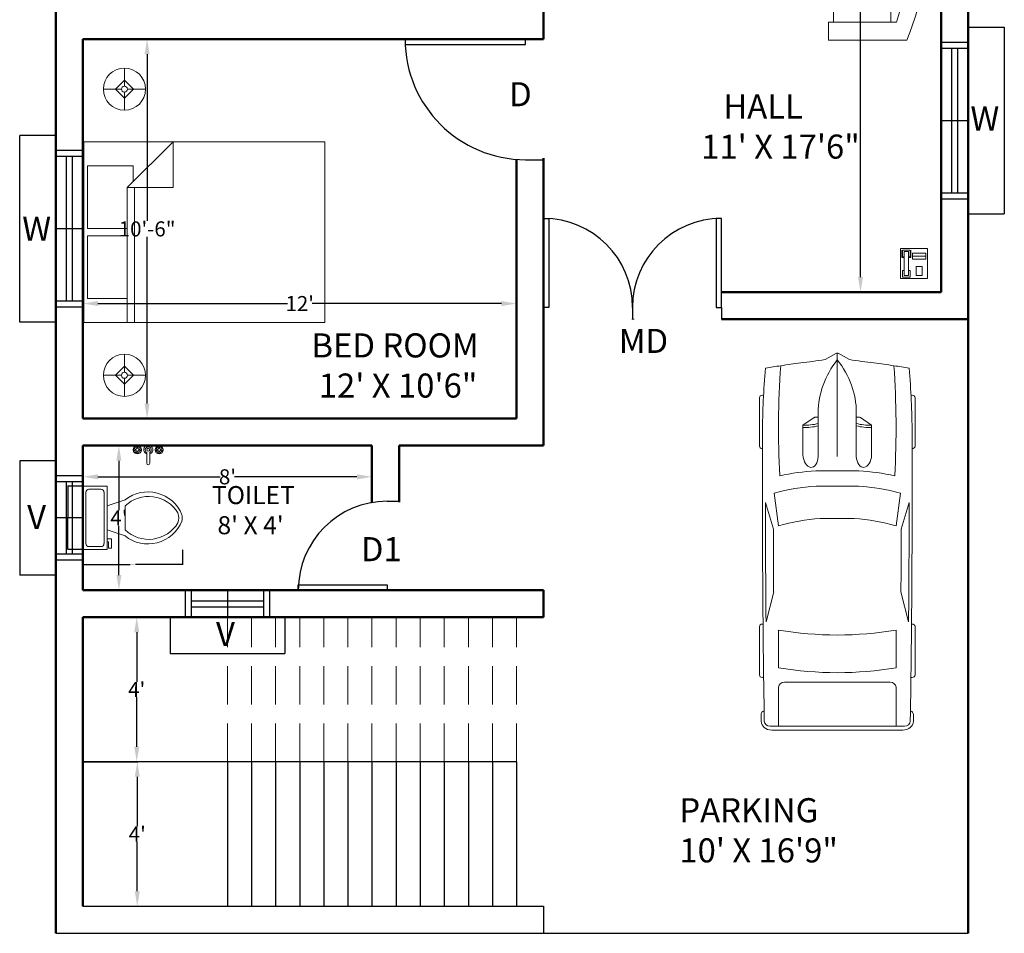
# Model space of a CAD drawing. Units: inches. Extents: x -25 to 789, y -921 to 230.
# Tile 2 of 5: x 5 to 332, y -315 to -11. Entities that reach past the tile are written whole.
import ezdxf

# ---------------------------------------------------------------- set-up
doc = ezdxf.new("R2010")
doc.units = ezdxf.units.IN
doc.header["$MEASUREMENT"] = 0
doc.linetypes.add('DASHED', pattern=[19.05, 12.7, -6.35])
for name, color, linetype, lineweight in [('A-ANNO-DIMS', 2, 'Continuous', 18), ('A-ANNO-TEXT', 7, 'Continuous', 18), ('A-AREA-IDEN', 3, 'Continuous', 18), ('A-DOOR', 4, 'Continuous', 25), ('A-FLOR-FIXT', 9, 'Continuous', 18), ('A-FLOR-OVHD', 8, 'DASHED', 18), ('A-FLOR-STRS', 3, 'Continuous', 25), ('A-FURN', 8, 'Continuous', 18), ('A-GLAZ', 4, 'Continuous', 25), ('A-WALL', 7, 'Continuous', 50), ('E-LITE-FIXT', 6, 'Continuous', 18), ('S-BEAM', 4, 'Continuous', 25)]:
    doc.layers.add(name, color=color, linetype=linetype, lineweight=lineweight)
doc.styles.get("Standard").update_dxf_attribs({"font": 'arial.ttf'})
doc.dimstyles.get("Standard").update_dxf_attribs({"dimtxt": 0.18, "dimasz": 0.18, "dimexe": 0.18, "dimexo": 0.0625, "dimgap": 0.09, "dimtad": 0, "dimtih": 1, "dimtoh": 1, "dimdec": 1, "dimzin": 0, "dimdsep": 46, "dimlunit": 4, "dimtxsty": 'Standard', "dimcen": 0.09, "dimadec": 0, "dimazin": 0, "dimtfac": 1, "dimtdec": 1, "dimtofl": 0, "dimtmove": 0, "dimatfit": 3, "dimfxl": 1, "dimtolj": 1, "dimtzin": 0, "dimarcsym": 0})

# ---------------------------------------------------------------- blocks, each defined once
blk = doc.blocks.new('*U2')
for p, q in [((0, 0), (0, -6)), ((-40, 0), (-40, -6))]:
    blk.add_line(p, q)
blk.add_lwpolyline([(0, 0), (0, 40), (-1.75, 40), (-1.75, 0)], close=True)
blk.add_arc((0, 0), 40, 90, 180)
blk = doc.blocks.new('Bed - Queen')
for p, q in [((0, -80.00003), (0, 0)), ((0, 0), (59.99999, 0)), ((59.99999, 0), (59.99999, -80.00003)), ((7.99999, -1.2), (28.79998, -1.2)), ((7.99999, -14.4), (7.99999, -1.2)), ((28.79998, -1.2), (28.79998, -14.4)), ((31.19999, -1.2), (51.99999, -1.2)), ((31.19999, -14.4), (31.19999, -1.2)), ((51.99999, -1.2), (51.99999, -16.4)), ((0, -14.4), (44.8, -14.4)), ((59.99999, -29.6), (44.8, -14.4)), ((44.8, -14.4), (44.8, -29.6)), ((44.8, -16.8), (0, -16.8)), ((51.99999, -16.4), (46.79936, -16.4)), ((44.8, -29.6), (59.99999, -29.6)), ((59.99999, -80.00003), (0, -80.00003))]:
    blk.add_line(p, q)
blk = doc.blocks.new('Lamp - Table')
for p, q in [((0, 7), (0, 1)), ((-1, 0), (-7, 0)), ((0, 3), (-3, 0)), ((-3, 0), (0, -3)), ((3, 0), (0, 3)), ((0, -3), (3, 0)), ((1, 0), (7, 0)), ((0, -1), (0, -7))]:
    blk.add_line(p, q)
for radius in [7, 1]:
    blk.add_circle((0, 0), radius)
blk = doc.blocks.new('Toilet - top')
for p, q in [((9.5, -6), (9.5, -2)), ((-10, -8.5), (-8, -8.5)), ((-10, -9.5), (-10, -8.5)), ((-7, -9.5), (-10, -9.5)), ((-8, -8.5), (-8, -8)), ((-7, -8), (-7, -9.5)), ((-4, -8), (-6, -14)), ((4, -8), (6, -14)), ((4, -14), (-4, -14))]:
    blk.add_line(p, q)
blk.add_lwpolyline([(10.5, -8), (10.5, 0), (-10.5, 0), (-10.5, -8)], close=True)
for points in [[(-9.5, -2), (-9.5, -6)], [(8.5, -1), (-8.5, -1)], [(-8.5, -7), (8.5, -7)]]:
    blk.add_lwpolyline(points)
for centre, radius, start, end in [((-8.62, -1.88), 0.884, 81.8699, 188.1301), ((8.62, -1.88), 0.884, 351.8699, 98.1301), ((-8.62, -6.12), 0.884, 171.8699, 278.1301), ((8.62, -6.12), 0.884, 261.8699, 8.1301), ((3.52, -21.58), 12.17, 141.4691, 247.9714), ((4.2, -21.82), 11.33, 136.3677, 238.9468), ((-3.52, -21.58), 12.17, 292.0284, 38.5307), ((-4.2, -21.82), 11.33, 301.053, 43.6321), ((0, -27.88), 4, 245.7318, 294.2682), ((0, -29), 4, 254.8605, 285.1395)]:
    blk.add_arc(centre, radius, start, end)
blk = doc.blocks.new('*U4')
for p, q in [((-750, 0), (-750, -100)), ((0, 0), (0, -100))]:
    blk.add_line(p, q)
blk.add_lwpolyline([(0, 0), (0, 750), (-43.75, 750), (-43.75, 0)], close=True)
blk.add_arc((0, 0), 750, 90, 180)
blk = doc.blocks.new('*U11')
for p, q in [((0, 0), (0, -100)), ((750, 0), (750, -100))]:
    blk.add_line(p, q)
blk.add_lwpolyline([(0, 0), (0, 750), (43.75, 750), (43.75, 0)], close=True)
blk.add_arc((0, 0), 750, 0, 90)
blk = doc.blocks.new('Phone - Desk')
for p, q in [((-4.5, -5), (-4.5, 5)), ((-4.5, 5), (4.5, 5)), ((-4, 4.5), (-4, 2)), ((-3.75, 4.5), (-3.75, 2.25)), ((-1.25, 4.5), (-3.75, 4.5)), ((-3.25, 4), (-3.25, -4)), ((-3.25, 4), (-1.75, 4)), ((-1.75, -4), (-1.75, 4)), ((-1.25, 2.25), (-1.25, 4.5)), ((-1, 2), (-1, 4.5)), ((4, 3.5), (-0.5, 3.5)), ((-0.5, 3.5), (-0.5, 1.5)), ((4, 1.5), (4, 3.5)), ((4.5, 5), (4.5, -5)), ((-4, 2), (-3.25, 2)), ((-3.75, 2.25), (-3.25, 2.25)), ((-1.75, 2.25), (-1.25, 2.25)), ((-1.75, 2), (-1, 2)), ((-0.5, 2.5), (4, 2.5)), ((-0.5, 1.5), (4, 1.5)), ((-3.75, -2.25), (-3.25, -2.25)), ((-3.75, -4.5), (-3.75, -2.25)), ((-1.75, -2.25), (-1.25, -2.25)), ((-1.25, -2.25), (-1.25, -4.5)), ((2.75, -1), (0.75, -1)), ((0.75, -1), (0.75, -4)), ((2.75, -4), (2.75, -1)), ((4.5, -5), (-4.5, -5)), ((-1.25, -4.5), (-3.75, -4.5)), ((-3.25, -4), (-1.75, -4)), ((0.75, -4), (2.75, -4))]:
    blk.add_line(p, q)
blk = doc.blocks.new('Sofa - Roundback 7 ft.')
for p, q in [((-12.00002, -32.4421), (-12.00003, -6.5971)), ((11.99997, -32.4421), (11.99998, -6.5971)), ((-36.000027, -34), (-36.000027, -11.4696)), ((35.99998, -34), (35.99998, -11.4696)), ((-35.999844, -13.3819), (35.9998, -13.3819)), ((-36.000027, -32.4421), (35.99998, -32.4421))]:
    blk.add_line(p, q)
for points in [[(-36.000027, -34), (-42.000027, -34), (-42.000027, -8)], [(41.99998, -8), (41.99998, -34), (35.99998, -34)]]:
    blk.add_lwpolyline(points)
for centre, radius, start, end in [((0, -114.25), 114.25, 68.43141, 111.5686), ((-0.00001, -127.1968), 121.1968, 72.72033, 107.2797)]:
    blk.add_arc(centre, radius, start, end)
blk = doc.blocks.new('*U19')
for p, q in [((21.1, 37.41), (21.1, 36.83)), ((46.55, 38.89), (22.35, 38.89)), ((47.8, 37.39), (47.8, 37.41)), ((87.99, 31.87), (74.76, 35.92)), ((134.31, 35.6), (119.29, 31.78)), ((135.45, 37.07), (135.45, 37.41)), ((136.7, 38.89), (160.9, 38.89)), ((162.15, 37.41), (162.15, 36.77)), ((70.03, 31.54), (86.41, 29.35)), ((186.47, -33.5), (186.47, 33.5)), ((188.4, -32.76), (188.4, 32.76)), ((138.42, 29.35), (157.25, 29.35)), ((164.52, 26.39), (164.52, -26.39)), ((186.47, 29.35), (167.01, 29.35)), ((32.27, 11.63), (36.13, 17.17)), ((36.13, 17.17), (50.94, 17.17)), ((32.12, 9.51), (32.12, 11.15)), ((58.92, -10.77), (58.92, 10.77)), ((66.55, -10.53), (66.55, 10.53)), ((186.47, -10.53), (186.47, 10.53)), ((3.27, 6.13), (0.1, 0.41)), ((29.77, 9.51), (51.68, 9.51)), ((82.74, 8.5), (82.74, -8.5)), ((0, 0), (51.68, 0)), ((0.1, -0.41), (3.27, -6.13)), ((29.77, -9.51), (51.68, -9.51)), ((32.12, -9.51), (32.12, -11.15)), ((32.27, -11.63), (36.13, -17.17)), ((36.13, -17.17), (50.94, -17.17)), ((86.41, -29.35), (70.03, -31.54)), ((157.25, -29.35), (138.42, -29.35)), ((167.01, -29.35), (186.47, -29.35)), ((87.99, -31.87), (74.76, -35.92)), ((134.31, -35.6), (119.29, -31.78)), ((21.1, -37.41), (21.1, -36.83)), ((46.55, -38.89), (22.35, -38.89)), ((47.8, -37.39), (47.8, -37.41)), ((135.45, -37.07), (135.45, -37.41)), ((136.7, -38.89), (160.9, -38.89)), ((162.15, -37.41), (162.15, -36.77))]:
    blk.add_line(p, q)
for centre, major_axis, ratio, start_param, end_param in [((266.03, -27.52), (0, 313.31), 0.842304, 1.367076, 1.39176), ((41.19, -490.86), (0, 528.23), 0.842304, 0.00281, 0.075598), ((22.35, 37.41), (0, -1.48), 0.842304, 3.141593, 4.712389), ((64.48, -10555.62), (0, 10593.03), 0.842304, -0.013397, 0.002797), ((46.55, 37.41), (0, 1.48), 0.842304, -1.570796, 0), ((64.48, -10555.62), (0, -10591.55), 0.842304, 3.133765, 3.140441), ((136.7, 37.41), (0, -1.48), 0.842304, 3.141593, 4.712389), ((160.9, 37.41), (0, 1.48), 0.842304, -1.570796, 0), ((180.63, 35.84), (0, 2.22), 0.842304, -0.013017, 1.249894), ((64.48, -10556.36), (0, 10595.31), 0.842304, -0.013397, -0.013017), ((183.98, 33.5), (0, -2.96), 0.842304, 1.570796, 3.128196), ((183.98, 32.76), (0, -5.25), 0.842304, 1.570796, 3.128196), ((37.47, -593.96), (0, -623.33), 0.842304, 3.096046, 3.200911), ((135.29, 5.39), (0, 81.77), 0.842304, 1.245306, 1.50788), ((95.79, -3666.35), (0, -3698.24), 0.842304, 3.134049, 3.144098), ((259.18, -27.52), (0, -305.3), 0.842304, 4.528606, 4.561838), ((134.4, 5.39), (0, -89.78), 0.842304, 4.449482, 4.652344), ((149.6, 2.8), (0, -79.58), 0.842304, 4.372215, 4.640744), ((17.08, 0), (0, 147.02), 0.842304, 4.511394, 4.913384), ((35.91, 0), (0, 147.02), 0.842304, 4.511394, 4.913384), ((167.01, 26.39), (0, 2.96), 0.842304, 0, 1.570796), ((-204.49, 52.4), (0, -250.96), 0.842304, 1.385369, 1.434372), ((13.04, 17.01), (0, 27.42), 0.842304, 4.435146, 4.718221), ((14.2, 17.01), (0, 27.42), 0.842304, 4.435146, 4.718221), ((50.79, 13.34), (6.34, -0.36), 0.603834, -1.395552, 1.581315), ((32.75, 11.15), (0, 0.74), 0.842304, 0.879714, 1.570796), ((29.77, -46.66), (0, 56.17), 0.842304, 0, 0.590319), ((0.62, 0), (0, -0.74), 0.842304, 4.131459, 5.293319), ((29.77, 46.66), (0, 56.17), 0.842304, 2.551274, 3.141593), ((-204.49, -52.4), (0, 250.96), 0.842304, -1.434372, -1.385369), ((13.04, -17.01), (0, -27.42), 0.842304, 1.564964, 1.848039), ((14.2, -17.01), (0, -27.42), 0.842304, 1.564964, 1.848039), ((149.6, -2.8), (0, -79.58), 0.842304, -1.499151, -1.230623), ((32.75, -11.15), (0, -0.74), 0.842304, 4.712389, 5.403472), ((134.4, -5.39), (0, -89.78), 0.842304, -1.510751, -1.307889), ((135.29, -5.39), (0, -81.77), 0.842304, -1.50788, -1.245306), ((259.18, 27.52), (0, 305.3), 0.842304, 1.721348, 1.754579), ((266.03, 27.52), (0, 313.31), 0.842304, 1.749832, 1.774517), ((37.47, 593.96), (0, -623.33), 0.842304, -0.059319, 0.045547), ((167.01, -26.39), (0, -2.96), 0.842304, 4.712389, 6.283185), ((95.79, 3666.35), (0, -3698.24), 0.842304, -0.002505, 0.007544), ((183.98, -33.5), (0, 2.96), 0.842304, 3.15499, 4.712389), ((183.98, -32.76), (0, -5.25), 0.842304, 0.013397, 1.570796), ((41.19, 490.86), (0, -528.23), 0.842304, -0.075598, -0.00281), ((22.35, -37.41), (0, 1.48), 0.842304, 1.570796, 3.141593), ((64.48, 10555.62), (0, 10593.03), 0.842304, 3.138796, 3.15499), ((46.55, -37.41), (0, -1.48), 0.842304, 0, 1.570796), ((64.48, 10555.62), (0, -10591.55), 0.842304, 0.001152, 0.007828), ((136.7, -37.41), (0, -1.48), 0.842304, -1.570796, 0), ((160.9, -37.41), (0, 1.48), 0.842304, 3.141593, 4.712389), ((180.63, -35.84), (0, -2.22), 0.842304, -1.249894, 0.013017), ((64.48, 10556.36), (0, 10595.31), 0.842304, 3.15461, 3.15499)]:
    blk.add_ellipse(centre, major_axis=major_axis, ratio=ratio, start_param=start_param, end_param=end_param)
at = {"extrusion": (0, 0, -1)}
blk.add_ellipse((50.79, -13.34), major_axis=(6.34, 0.36), ratio=0.603834, start_param=-1.395552, end_param=1.581315, dxfattribs=at)
blk = doc.blocks.new('*U20')
for p, q in [((-750, 0), (-750, 100)), ((0, 0), (0, 100))]:
    blk.add_line(p, q)
blk.add_lwpolyline([(0, 0), (0, -750), (-43.75, -750), (-43.75, 0)], close=True)
blk.add_arc((0, 0), 750, 180, 270)
blk = doc.blocks.new('Faucet - Bathroom top')
for p, q in [((-4.107, 0.125), (-4.375, 0.125)), ((-3.75, 0.4788), (-3.75, 0.75)), ((-3.5, 0.482), (-3.5, 0.75)), ((-3.1461, 0.125), (-2.875, 0.125)), ((3.143, 0.125), (2.875, 0.125)), ((3.5, 0.4788), (3.5, 0.75)), ((3.75, 0.482), (3.75, 0.75)), ((4.1039, 0.125), (4.375, 0.125)), ((-4.1039, -0.125), (-4.375, -0.125)), ((-3.75, -0.4821), (-3.75, -0.75)), ((-3.5, -0.4789), (-3.5, -0.75)), ((-3.143, -0.125), (-2.875, -0.125)), ((-0.5, -0.8639), (-0.5, -4.5)), ((0.5, -4.5), (0.5, -0.8631)), ((3.1461, -0.125), (2.875, -0.125)), ((3.5, -0.4821), (3.5, -0.75)), ((3.75, -0.4789), (3.75, -0.75)), ((4.107, -0.125), (4.375, -0.125))]:
    blk.add_line(p, q)
for centre, radius in [((-3.625, 0), 1.375), ((-4.625, 0), 0.2795), ((-3.625, 0), 0.5), ((-3.625, 1), 0.2795), ((-2.625, 0), 0.2795), ((0, 0), 0.5), ((3.625, 0), 1.375), ((2.625, 0), 0.2795), ((3.625, 0), 0.5), ((3.625, 1), 0.2795), ((4.625, 0), 0.2795), ((-3.625, -1), 0.2795), ((3.625, -1), 0.2795)]:
    blk.add_circle(centre, radius)
for centre, radius, start, end in [((-3.625, 0), 1, 105.2407, 164.2093), ((-3.625, 0), 1, 16.44125, 74.07887), ((0, 0), 1.5, 289.6514, 250.3603), ((0, 0), 1, 300.3431, 239.7554), ((3.625, 0), 1, 106.12, 164.0884), ((3.625, 0), 1, 16.23422, 73.90469), ((-3.625, 0), 1, 196.2342, 253.9047), ((-3.625, 0), 1, 286.12, 344.0884), ((3.625, 0), 1, 196.4413, 254.0789), ((3.625, 0), 1, 285.2407, 344.2093), ((0, -4.5), 0.5, 180, 0)]:
    blk.add_arc(centre, radius, start, end)
blk = doc.blocks.new('*D47')
at = {"layer": 'A-ANNO-DIMS', "color": 0, "lineweight": -2, "transparency": 16777216}
for p, q in [((26.26, -153.04), (26.26, -163.51)), ((122.26, -153.04), (122.26, -163.51)), ((31.26, -163.33), (71.87, -163.33)), ((117.26, -163.33), (76.65, -163.33))]:
    blk.add_line(p, q, dxfattribs=at)
at = {"layer": 'A-ANNO-DIMS', "color": 0, "transparency": 16777216}
for points in [[(31.26, -162.5), (31.26, -164.17), (26.26, -163.33)], [(117.26, -162.5), (117.26, -164.17), (122.26, -163.33)]]:
    blk.add_solid(points, dxfattribs=at)
at = {"layer": 'Defpoints', "color": 0, "transparency": 16777216}
for p in [(26.26, -152.98), (122.26, -152.98), (122.26, -163.33)]:
    blk.add_point(p, dxfattribs=at)
at = {"layer": 'A-ANNO-DIMS', "color": 0, "transparency": 16777216, "insert": (74.26, -163.33), "char_height": 5, "attachment_point": 5}
blk.add_mtext("\\A1;8'", dxfattribs=at)
blk = doc.blocks.new('*D48')
at = {"layer": 'A-ANNO-DIMS', "color": 0, "lineweight": -2, "transparency": 16777216}
for p, q in [((26.32, -152.98), (38.39, -152.98)), ((38.21, -157.98), (38.21, -174.39)), ((38.21, -195.98), (38.21, -179.57)), ((26.32, -200.98), (38.39, -200.98))]:
    blk.add_line(p, q, dxfattribs=at)
at = {"layer": 'A-ANNO-DIMS', "color": 0, "transparency": 16777216}
for points in [[(37.38, -157.98), (39.04, -157.98), (38.21, -152.98)], [(37.38, -195.98), (39.04, -195.98), (38.21, -200.98)]]:
    blk.add_solid(points, dxfattribs=at)
at = {"layer": 'Defpoints', "color": 0, "transparency": 16777216}
for p in [(26.26, -152.98), (26.26, -200.98), (38.21, -200.98)]:
    blk.add_point(p, dxfattribs=at)
at = {"layer": 'A-ANNO-DIMS', "color": 0, "transparency": 16777216, "insert": (38.21, -176.98), "char_height": 5, "attachment_point": 5}
blk.add_mtext("\\A1;4'", dxfattribs=at)
blk = doc.blocks.new('*D49')
at = {"layer": 'A-ANNO-DIMS', "color": 0, "lineweight": -2, "transparency": 16777216}
for p, q in [((26.32, -17.98), (47.75, -17.98)), ((47.57, -22.98), (47.57, -78.34)), ((47.57, -138.98), (47.57, -83.62)), ((26.32, -143.98), (47.75, -143.98))]:
    blk.add_line(p, q, dxfattribs=at)
at = {"layer": 'A-ANNO-DIMS', "color": 0, "transparency": 16777216}
for points in [[(46.73, -22.98), (48.4, -22.98), (47.57, -17.98)], [(46.73, -138.98), (48.4, -138.98), (47.57, -143.98)]]:
    blk.add_solid(points, dxfattribs=at)
at = {"layer": 'Defpoints', "color": 0, "transparency": 16777216}
for p in [(26.26, -17.98), (26.26, -143.98), (47.57, -143.98)]:
    blk.add_point(p, dxfattribs=at)
at = {"layer": 'A-ANNO-DIMS', "color": 0, "transparency": 16777216, "insert": (47.57, -80.98), "char_height": 5, "attachment_point": 5}
blk.add_mtext('\\A1;10\'-6"', dxfattribs=at)
blk = doc.blocks.new('*D50')
at = {"layer": 'A-ANNO-DIMS', "color": 0, "lineweight": -2, "transparency": 16777216}
for p, q in [((26.26, -143.92), (26.26, -105.6)), ((31.26, -105.78), (94.16, -105.78)), ((165.26, -105.78), (102.36, -105.78)), ((170.26, -143.92), (170.26, -105.6))]:
    blk.add_line(p, q, dxfattribs=at)
at = {"layer": 'A-ANNO-DIMS', "color": 0, "transparency": 16777216}
for points in [[(31.26, -104.95), (31.26, -106.61), (26.26, -105.78)], [(165.26, -104.95), (165.26, -106.61), (170.26, -105.78)]]:
    blk.add_solid(points, dxfattribs=at)
at = {"layer": 'Defpoints', "color": 0, "transparency": 16777216}
for p in [(170.26, -105.78), (26.26, -143.98), (170.26, -143.98)]:
    blk.add_point(p, dxfattribs=at)
at = {"layer": 'A-ANNO-DIMS', "color": 0, "transparency": 16777216, "insert": (98.26, -105.78), "char_height": 5, "attachment_point": 5}
blk.add_mtext("\\A1;12'", dxfattribs=at)
blk = doc.blocks.new('*D56')
at = {"layer": 'A-ANNO-DIMS', "color": 0, "lineweight": -2, "transparency": 16777216}
for p, q in [((311.2, 108.02), (284.32, 108.02)), ((284.5, 103.02), (284.5, 5.66)), ((284.5, -96.98), (284.5, 0.38)), ((311.2, -101.98), (284.32, -101.98))]:
    blk.add_line(p, q, dxfattribs=at)
at = {"layer": 'A-ANNO-DIMS', "color": 0, "transparency": 16777216}
for points in [[(283.67, 103.02), (285.33, 103.02), (284.5, 108.02)], [(283.67, -96.98), (285.33, -96.98), (284.5, -101.98)]]:
    blk.add_solid(points, dxfattribs=at)
at = {"layer": 'Defpoints', "color": 0, "transparency": 16777216}
for p in [(284.5, 108.02), (311.26, 108.02), (311.26, -101.98)]:
    blk.add_point(p, dxfattribs=at)
at = {"layer": 'A-ANNO-DIMS', "color": 0, "transparency": 16777216, "insert": (284.5, 3.02), "char_height": 5, "attachment_point": 5}
blk.add_mtext('\\A1;17\'-6"', dxfattribs=at)
blk = doc.blocks.new('*D57')
at = {"layer": 'A-ANNO-DIMS', "color": 0, "lineweight": -2, "transparency": 16777216}
for p, q in [((26.32, -209.98), (44.31, -209.98)), ((44.13, -214.98), (44.13, -231.39)), ((44.13, -252.98), (44.13, -236.57)), ((26.32, -257.98), (44.31, -257.98))]:
    blk.add_line(p, q, dxfattribs=at)
at = {"layer": 'A-ANNO-DIMS', "color": 0, "transparency": 16777216}
for points in [[(43.3, -214.98), (44.97, -214.98), (44.13, -209.98)], [(43.3, -252.98), (44.97, -252.98), (44.13, -257.98)]]:
    blk.add_solid(points, dxfattribs=at)
at = {"layer": 'Defpoints', "color": 0, "transparency": 16777216}
for p in [(26.26, -209.98), (44.13, -209.98), (26.26, -257.98)]:
    blk.add_point(p, dxfattribs=at)
at = {"layer": 'A-ANNO-DIMS', "color": 0, "transparency": 16777216, "insert": (44.13, -233.98), "char_height": 5, "attachment_point": 5}
blk.add_mtext("\\A1;4'", dxfattribs=at)
blk = doc.blocks.new('*D58')
at = {"layer": 'A-ANNO-DIMS', "color": 0, "lineweight": -2, "transparency": 16777216}
for p, q in [((26.32, -257.98), (44.49, -257.98)), ((44.31, -262.98), (44.31, -279.39)), ((44.31, -300.98), (44.31, -284.57)), ((26.32, -305.98), (44.49, -305.98))]:
    blk.add_line(p, q, dxfattribs=at)
at = {"layer": 'A-ANNO-DIMS', "color": 0, "transparency": 16777216}
for points in [[(43.48, -262.98), (45.15, -262.98), (44.31, -257.98)], [(43.48, -300.98), (45.15, -300.98), (44.31, -305.98)]]:
    blk.add_solid(points, dxfattribs=at)
at = {"layer": 'Defpoints', "color": 0, "transparency": 16777216}
for p in [(26.26, -257.98), (44.31, -257.98), (26.26, -305.98)]:
    blk.add_point(p, dxfattribs=at)
at = {"layer": 'A-ANNO-DIMS', "color": 0, "transparency": 16777216, "insert": (44.31, -281.98), "char_height": 5, "attachment_point": 5}
blk.add_mtext("\\A1;4'", dxfattribs=at)
blk = doc.blocks.new('WIN-W-SUNSHADE')
at = {"ltscale": 2}
for p, q in [((0, 9), (0, 21)), ((0, 21), (62, 21)), ((62, 9), (62, 21)), ((5, 9), (0, 9)), ((57, 9), (62, 9))]:
    blk.add_line(p, q, dxfattribs=at)
for p, q in [((5, 0), (5, 9)), ((57, 0), (57, 9))]:
    blk.add_line(p, q)
blk = doc.blocks.new('WIN-V-SUNSHADE')
for p, q in [((0, 9), (0, 21)), ((38, 21), (0, 21)), ((38, 9), (38, 21)), ((5, 9), (0, 9)), ((5, 0), (5, 9)), ((33, 0), (33, 9)), ((33, 9), (38, 9))]:
    blk.add_line(p, q)
blk = doc.blocks.new('*D87')
at = {"layer": 'A-ANNO-DIMS', "color": 0, "lineweight": -2, "transparency": 16777216}
for p, q in [((26.26, -187.54), (26.26, -192.61)), ((59.31, -187.54), (59.31, -192.61)), ((26.44, -192.43), (41.9, -192.43)), ((59.13, -192.43), (43.67, -192.43))]:
    blk.add_line(p, q, dxfattribs=at)
at = {"layer": 'A-ANNO-DIMS', "color": 0, "transparency": 16777216}
for points in [[(26.44, -192.4), (26.44, -192.46), (26.26, -192.43)], [(59.13, -192.4), (59.13, -192.46), (59.31, -192.43)]]:
    blk.add_solid(points, dxfattribs=at)
at = {"layer": 'Defpoints', "color": 0, "transparency": 16777216}
for p in [(26.26, -187.48), (59.31, -187.48), (26.26, -192.43)]:
    blk.add_point(p, dxfattribs=at)
at = {"layer": 'A-ANNO-DIMS', "color": 0, "transparency": 16777216, "insert": (42.78, -192.43), "char_height": 0.18, "attachment_point": 5}
blk.add_mtext('\\A1;WC 2\'-9" TYP.', dxfattribs=at)
blk = doc.blocks.new('*D88')
at = {"layer": 'A-ANNO-DIMS', "color": 0, "lineweight": -2, "transparency": 16777216}
for p, q in [((26.2, -166.48), (21.12, -166.48)), ((21.3, -166.66), (21.3, -176.8)), ((21.3, -187.3), (21.3, -177.16)), ((26.2, -187.48), (21.12, -187.48))]:
    blk.add_line(p, q, dxfattribs=at)
at = {"layer": 'A-ANNO-DIMS', "color": 0, "transparency": 16777216}
for points in [[(21.27, -166.66), (21.33, -166.66), (21.3, -166.48)], [(21.27, -187.3), (21.33, -187.3), (21.3, -187.48)]]:
    blk.add_solid(points, dxfattribs=at)
at = {"layer": 'Defpoints', "color": 0, "transparency": 16777216}
for p in [(21.3, -166.48), (26.26, -166.48), (26.26, -187.48)]:
    blk.add_point(p, dxfattribs=at)
at = {"layer": 'A-ANNO-DIMS', "color": 0, "transparency": 16777216, "insert": (21.3, -176.98), "char_height": 0.18, "attachment_point": 5}
blk.add_mtext('\\A1;1\'-9" TYP.', dxfattribs=at)

msp = doc.modelspace()

# ---------------------------------------------------------------- linework, layer by layer
at = {"layer": 'A-FLOR-OVHD'}
for p, q in [((74.26, -257.98), (74.26, -209.98)), ((82.26, -257.98), (82.26, -209.98)), ((90.26, -257.98), (90.26, -209.98)), ((98.26, -257.98), (98.26, -209.98)), ((106.26, -257.98), (106.26, -209.98)), ((114.26, -257.98), (114.26, -209.98)), ((122.26, -257.98), (122.26, -209.98)), ((130.26, -257.98), (130.26, -209.98)), ((138.26, -257.98), (138.26, -209.98)), ((146.26, -257.98), (146.26, -209.98)), ((154.26, -257.98), (154.26, -209.98)), ((162.26, -257.98), (162.26, -209.98)), ((170.26, -257.98), (170.26, -209.98))]:
    msp.add_line(p, q, dxfattribs=at)
at = {"layer": 'A-FLOR-STRS'}
for p, q in [((170.26, -257.98), (26.26, -257.98)), ((74.26, -257.98), (74.26, -305.98)), ((82.26, -257.98), (82.26, -305.98)), ((90.26, -257.98), (90.26, -305.98)), ((98.26, -257.98), (98.26, -305.98)), ((106.26, -257.98), (106.26, -305.98)), ((114.26, -257.98), (114.26, -305.98)), ((122.26, -257.98), (122.26, -305.98)), ((130.26, -257.98), (130.26, -305.98)), ((138.26, -257.98), (138.26, -305.98)), ((146.26, -257.98), (146.26, -305.98)), ((154.26, -257.98), (154.26, -305.98)), ((162.26, -257.98), (162.26, -305.98)), ((170.26, -257.98), (170.26, -305.98))]:
    msp.add_line(p, q, dxfattribs=at)
at = {"layer": 'A-FURN'}
msp.add_line((209.38, -110.98), (208.52, -110.98), dxfattribs=at)
at = {"layer": 'A-GLAZ'}
for p, q in [((311.26, -20.98), (320.26, -20.98)), ((314.76, -20.98), (314.76, -68.98)), ((316.76, -20.98), (316.76, -68.98)), ((311.26, -44.98), (320.26, -44.98)), ((26.26, -56.98), (17.26, -56.98)), ((20.76, -104.98), (20.76, -56.98)), ((22.76, -104.98), (22.76, -56.98)), ((311.26, -68.98), (320.26, -68.98)), ((26.26, -80.98), (17.26, -80.98)), ((26.26, -104.98), (17.26, -104.98)), ((26.26, -164.98), (17.26, -164.98)), ((20.76, -188.98), (20.76, -164.98)), ((22.76, -188.98), (22.76, -164.98)), ((26.26, -176.98), (17.26, -176.98)), ((26.26, -188.98), (17.26, -188.98)), ((62.26, -200.98), (62.26, -209.98)), ((74.26, -200.98), (74.26, -209.98)), ((86.26, -200.98), (86.26, -209.98)), ((62.26, -204.48), (86.26, -204.48)), ((62.26, -206.48), (86.26, -206.48))]:
    msp.add_line(p, q, dxfattribs=at)
at = {"layer": 'A-WALL'}
for p, q in [((17.26, -17.98), (17.26, 174.02)), ((311.26, 108.02), (311.26, -101.98)), ((320.26, 108.02), (320.26, -314.98)), ((179.26, -17.98), (179.26, 68.02)), ((17.26, -17.98), (17.26, -152.98)), ((26.26, -17.98), (179.26, -17.98)), ((26.26, -17.98), (26.26, -143.98)), ((170.26, -143.98), (170.26, -57.87)), ((179.26, -110.98), (179.26, -57.53)), ((311.26, -101.98), (238.31, -101.98)), ((179.26, -152.98), (179.26, -110.98)), ((320.26, -110.98), (238.31, -110.98)), ((26.26, -143.98), (170.26, -143.98)), ((17.26, -152.98), (17.26, -209.98)), ((26.26, -152.98), (122.26, -152.98)), ((26.26, -152.98), (26.26, -200.98)), ((122.26, -171.89), (122.26, -152.98)), ((131.26, -171.71), (131.26, -152.98)), ((131.26, -152.98), (179.26, -152.98)), ((26.26, -200.98), (131.26, -200.98)), ((131.26, -200.98), (179.26, -200.98)), ((179.26, -209.98), (179.26, -200.98)), ((17.26, -209.98), (17.26, -314.98)), ((26.26, -209.98), (179.26, -209.98)), ((26.26, -209.98), (26.26, -305.98))]:
    msp.add_line(p, q, dxfattribs=at)
at = {"layer": 'S-BEAM'}
for p, q in [((26.26, -305.98), (179.26, -305.98)), ((179.26, -305.98), (179.26, -314.98)), ((17.26, -314.98), (320.26, -314.98))]:
    msp.add_line(p, q, dxfattribs=at)

# ---------------------------------------------------------------- block references
at = {"layer": 'A-DOOR', "rotation": 90}
msp.add_blockref('*U2', (173.26, -17.98), dxfattribs=at)
at = {"layer": 'A-DOOR', "xscale": 0.0393700787401575, "yscale": 0.0393700787401575, "zscale": 0.0393700787401575}
for name, p in [('*U11', (179.26, -107.04)), ('*U4', (238.31, -107.04))]:
    msp.add_blockref(name, p, dxfattribs=at)
at = {"layer": 'A-DOOR', "xscale": 0.0393700787401575, "yscale": 0.0393700787401575, "zscale": 0.0393700787401575, "rotation": 270}
msp.add_blockref('*U20', (127.32, -200.98), dxfattribs=at)
at = {"layer": 'A-FLOR-FIXT'}
msp.add_blockref('Faucet - Bathroom top', (47.95, -154.34), dxfattribs=at)
at = {"layer": 'A-FLOR-FIXT', "rotation": 90}
msp.add_blockref('Toilet - top', (26.26, -176.98), dxfattribs=at)
at = {"layer": 'A-FURN'}
for name, p, rotation in [('Sofa - Roundback 7 ft.', (307.92, 23.71), 270), ('Bed - Queen', (26.58, -112.07), 90)]:
    msp.add_blockref(name, p, dxfattribs=dict(at, rotation=rotation))
msp.add_blockref('Phone - Desk', (302.23, -92.5), dxfattribs=at)
at = {"layer": 'A-FURN', "xscale": 0.6647672135432005, "yscale": 0.6647672135432005, "zscale": 0.6647672135432005, "rotation": 270}
msp.add_blockref('*U19', (276.79, -122.21), dxfattribs=at)
at = {"layer": 'A-GLAZ'}
for name, p, rotation in [('WIN-W-SUNSHADE', (311.26, -13.98), 270.0000000000001), ('WIN-W-SUNSHADE', (26.26, -111.98), 90.00000000000026), ('WIN-V-SUNSHADE', (26.26, -195.98), 89.99999999999969), ('WIN-V-SUNSHADE', (93.26, -200.98), 180)]:
    msp.add_blockref(name, p, dxfattribs=dict(at, rotation=rotation))
at = {"layer": 'E-LITE-FIXT'}
for p in [(40.05, -34.55), (40.05, -129.61)]:
    msp.add_blockref('Lamp - Table', p, dxfattribs=at)

# ---------------------------------------------------------------- texts
at = {"layer": 'A-ANNO-TEXT'}
for s, p in [('D', (167.81, -40.24)), ('W', (321, -48.29)), ('W', (6.1, -84.93)), ('MD', (204.23, -122.19)), ('V', (7.74, -180.69)), ('D1', (118.57, -191.37)), ('V', (70.46, -219.58))]:
    msp.add_text(s, height=8, dxfattribs=at).set_placement(p)
at = {"layer": 'A-AREA-IDEN', "attachment_point": 1}
for s, insert, char_height in [('   HALL \\P11\' X 17\'6"', (231.6, -36.31), 8), ('BED ROOM\\P 12\' X 10\'6"', (102.15, -115.68), 8), ("TOILET\\P 8' X 4'", (69.11, -166.41), 6), ('PARKING\\P10\' X 16\'9"', (224.34, -270.09), 8)]:
    msp.add_mtext_dynamic_manual_height_columns(s, width=99.8363, gutter_width=1, heights=[0], dxfattribs=dict(at, insert=insert, char_height=char_height))

# ---------------------------------------------------------------- dimensions: what is measured, and where the dimension line sits
at = {"layer": 'A-ANNO-DIMS'}
for base, p1, p2, picture, middle in [((284.5, 108.02), (311.26, -101.98), (311.26, 108.02), '*D56', (284.5, 3.02)), ((47.57, -143.98), (26.26, -17.98), (26.26, -143.98), '*D49', (47.57, -80.98)), ((38.21, -200.98), (26.26, -152.98), (26.26, -200.98), '*D48', (38.21, -176.98)), ((44.13, -209.98), (26.26, -257.98), (26.26, -209.98), '*D57', (44.13, -233.98)), ((44.31, -257.98), (26.26, -305.98), (26.26, -257.98), '*D58', (44.31, -281.98))]:
    dim = msp.add_linear_dim(base=base, p1=p1, p2=p2, angle=90, dimstyle='Standard', override={"dimtxt": 5, "dimasz": 5, "dimclrd": 0, "dimclre": 0, "dimclrt": 0}, dxfattribs=at)
    dim.commit()
    dim.dimension.update_dxf_attribs({"geometry": picture, "text_midpoint": middle})
for base, p1, p2, picture, middle in [((170.26, -105.78), (26.26, -143.98), (170.26, -143.98), '*D50', (98.26, -105.78)), ((122.26, -163.33), (26.26, -152.98), (122.26, -152.98), '*D47', (74.26, -163.33))]:
    dim = msp.add_linear_dim(base=base, p1=p1, p2=p2, dimstyle='Standard', override={"dimtxt": 5, "dimasz": 5, "dimclrd": 0, "dimclre": 0, "dimclrt": 0}, dxfattribs=at)
    dim.commit()
    dim.dimension.update_dxf_attribs({"geometry": picture, "text_midpoint": middle})
for base, p1, p2, angle, text, picture, middle in [((21.3, -166.48), (26.26, -187.48), (26.26, -166.48), 90, '<> TYP.', '*D88', (21.3, -176.98)), ((26.2594, -192.435), (59.3057, -187.4781), (26.2594, -187.4781), 180, 'WC <> TYP.', '*D87', (42.7825, -192.435))]:
    dim = msp.add_linear_dim(base=base, p1=p1, p2=p2, angle=angle, text=text, dimstyle='Standard', override={"dimdec": 1, "dimrnd": 0, "dimzin": 1, "dimlunit": 4, "dimfrac": 2}, dxfattribs=at)
    dim.commit()
    dim.dimension.update_dxf_attribs({"geometry": picture, "text_midpoint": middle})

doc.saveas('drawing.dxf')
